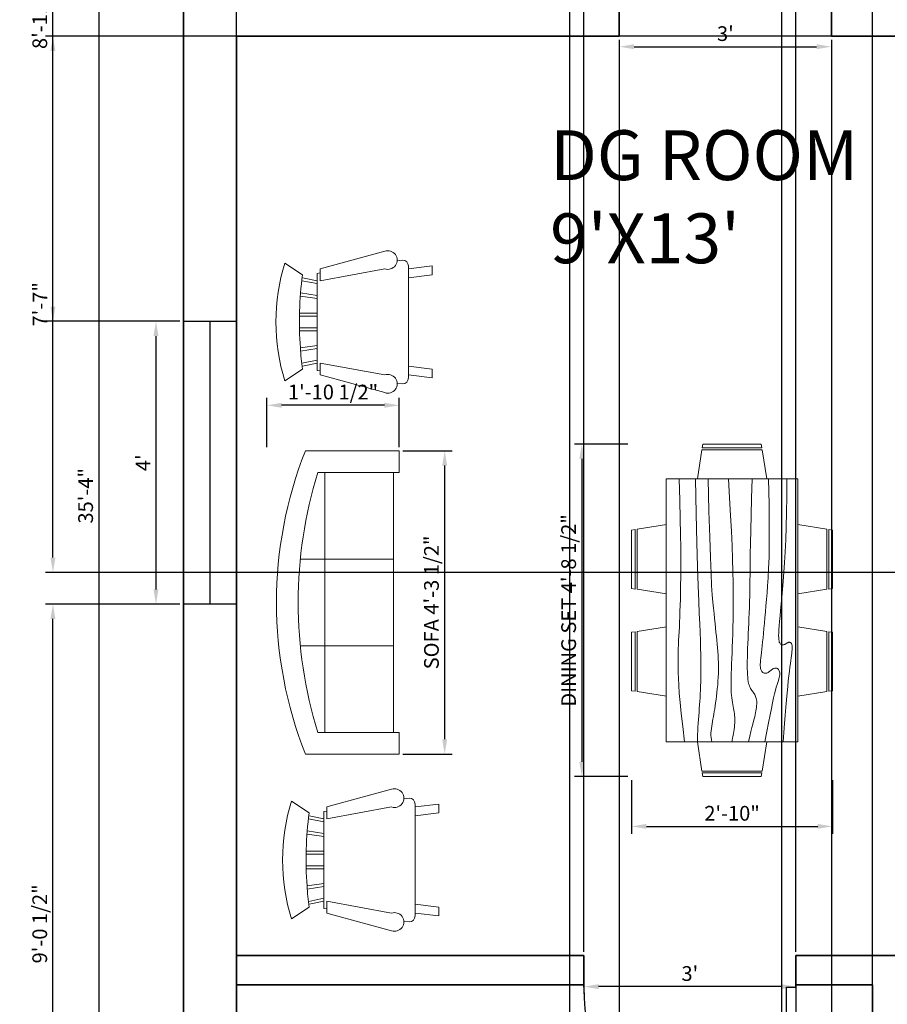
# Model space of a CAD drawing. Units: inches. Extents: x 2459 to 2755, y 1300 to 1776.
# Tile 2 of 4: x 2459 to 2606, y 1450 to 1617. Entities that reach past the tile are written whole.
import ezdxf

# ---------------------------------------------------------------- set-up
doc = ezdxf.new("R2010")
doc.units = ezdxf.units.IN
for name, color, linetype, lineweight in [('A-AREA-IDEN', 3, 'Continuous', 25), ('A-WALL', 7, 'Continuous', 35), ('DIM', 4, 'Continuous', 18), ('DOOR', 20, 'Continuous', 25), ('FURNITURE', 6, 'Continuous', 18), ('WIN', 2, 'Continuous', 25)]:
    doc.layers.add(name, color=color, linetype=linetype, lineweight=lineweight)
doc.styles.get("Standard").update_dxf_attribs({"font": 'arial.ttf'})
doc.dimstyles.new('ISO-25', dxfattribs={"dimtxt": 2.5, "dimasz": 2.5, "dimexe": 1.25, "dimexo": 0.625, "dimtad": 1, "dimlunit": 3, "dimtxsty": 'Standard', "dimcen": 2.5, "dimadec": 0, "dimazin": 0, "dimtfac": 1, "dimtmove": 0, "dimatfit": 3, "dimfxl": 1, "dimarcsym": 0})

# ---------------------------------------------------------------- blocks, each defined once
blk = doc.blocks.new('*U3')
for p, q in [((0, 0), (0, -6)), ((-40, 0), (-40, -6))]:
    blk.add_line(p, q)
blk.add_lwpolyline([(0, 0), (0, 40), (-1.75, 40), (-1.75, 0)], close=True)
blk.add_arc((0, 0), 40, 90, 180)
blk = doc.blocks.new('*U4')
for p, q in [((-40, 0), (-40, 6)), ((0, 0), (0, 6))]:
    blk.add_line(p, q)
blk.add_lwpolyline([(0, 0), (0, -40), (-1.75, -40), (-1.75, 0)], close=True)
blk.add_arc((0, 0), 40, 180, 270)
blk = doc.blocks.new('Dining Set - 36 x 72 in.')
for p, q in [((-22, 27.5), (-22.1562, 26.50042)), ((-22, 27.5), (-6, 27.5)), ((-5.8437, 26.49966), (-6, 27.5)), ((6, 27.5), (5.8438, 26.50042)), ((6, 27.5), (22, 27.5)), ((22.1563, 26.49966), (22, 27.5)), ((-22.2343, 26.00059), (-23.4847, 17.99762)), ((-22.2304, 26), (-5.7608, 26)), ((-5.8416, 26.5), (-22.1534, 26.5)), ((-4.5152, 17.99762), (-5.7655, 25.99926)), ((5.7657, 26.00059), (4.5153, 17.99762)), ((5.7696, 26), (22.2392, 26)), ((22.1584, 26.5), (5.8466, 26.5)), ((23.4848, 17.99762), (22.2345, 25.99926)), ((36, 18), (-36, 18)), ((-36, 18), (-36, -18)), ((36, -18), (36, 18)), ((-45.5, 8), (-44.5004, 8.15617)), ((-44.5, -8.15843), (-44.5, 8.15338)), ((-44.0006, 8.23428), (-35.9976, 9.48474)), ((-44, 8.23041), (-44, -8.23915)), ((44.0006, 8.23428), (35.9976, 9.48474)), ((44, 8.23041), (44, -8.23915)), ((44.5, -8.15843), (44.5, 8.15338)), ((45.5, 8), (44.5005, 8.15617)), ((-45.5, 8), (-45.5, -8)), ((45.5, 8), (45.5, -8)), ((-44.4997, -8.15631), (-45.5, -8)), ((44.4997, -8.15631), (45.5, -8)), ((-35.9976, -9.48476), (-43.9993, -8.2345)), ((35.9976, -9.48476), (43.9993, -8.2345)), ((-36, -18), (36, -18)), ((-22.2343, -26.0006), (-23.4847, -17.99762)), ((-4.5152, -17.99762), (-5.7655, -25.99928)), ((5.7657, -26.0006), (4.5153, -17.99762)), ((23.4848, -17.99762), (22.2345, -25.99928)), ((-22.2304, -26), (-5.7608, -26)), ((-22, -27.5), (-22.1562, -26.50044)), ((-5.8416, -26.5), (-22.1534, -26.5)), ((-5.8437, -26.49967), (-6, -27.5)), ((5.7696, -26), (22.2392, -26)), ((6, -27.5), (5.8438, -26.50044)), ((22.1584, -26.5), (5.8466, -26.5)), ((22.1563, -26.49967), (22, -27.5)), ((-22, -27.5), (-6, -27.5)), ((6, -27.5), (22, -27.5))]:
    blk.add_line(p, q)
for points in [[(-36, 15), (-31.1772, 14.97754), (-26.8079, 14.91406), (-22.8538, 14.81543), (-19.276, 14.6875), (-16.0362, 14.53613), (-13.0957, 14.36718), (-10.4159, 14.18652), (-7.9583, 14), (-5.6904, 13.81315), (-3.6035, 13.63021), (-1.6954, 13.45508), (0.0365, 13.29166), (1.5945, 13.14388), (2.9811, 13.01562), (4.1988, 12.9108), (5.25, 12.83333), (6.1393, 12.78613), (6.8802, 12.76823), (7.4883, 12.77767), (7.9792, 12.8125), (8.3685, 12.87077), (8.6719, 12.95052), (8.9049, 13.0498), (9.0833, 13.16666), (9.2205, 13.29899), (9.3216, 13.44401), (9.3895, 13.59879), (9.4271, 13.76041), (9.4373, 13.92594), (9.4232, 14.09245), (9.3875, 14.257), (9.3333, 14.41666), (9.2638, 14.56917), (9.1836, 14.71484), (9.0975, 14.85465), (9.0104, 14.98958), (8.9272, 15.1206), (8.8529, 15.2487), (8.7922, 15.37483), (8.75, 15.5), (8.7305, 15.62467), (8.7344, 15.74739), (8.7617, 15.86621), (8.8125, 15.97916), (8.8867, 16.08431), (8.9844, 16.17968), (9.1055, 16.26334), (9.25, 16.33333), (9.4189, 16.38802), (9.6172, 16.42708), (9.8506, 16.45052), (10.125, 16.45833), (10.4463, 16.45052), (10.8203, 16.42708), (11.2529, 16.38802), (11.75, 16.33333), (12.3184, 16.26318), (12.9694, 16.17838), (13.7151, 16.07991), (14.5677, 15.96875), (15.5395, 15.84586), (16.6426, 15.71224), (17.8893, 15.56884), (19.2917, 15.41666), (20.859, 15.25667), (22.5879, 15.08984), (24.4721, 14.91715), (26.5052, 14.73958), (28.6809, 14.5581), (30.9929, 14.3737), (33.4347, 14.18733), (36, 14)], [(-36, 10), (-28.9766, 10.14274), (-23.1725, 10.20442), (-18.4241, 10.19775), (-14.5677, 10.13541), (-11.4399, 10.03011), (-8.877, 9.89453), (-6.7154, 9.74137), (-4.7917, 9.58333), (-2.9698, 9.43082), (-1.2246, 9.28515), (0.4415, 9.14534), (2.026, 9.01041), (3.5266, 8.87939), (4.9408, 8.7513), (6.266, 8.62516), (7.5, 8.5), (8.6411, 8.37549), (9.6914, 8.2539), (10.6538, 8.13818), (11.5312, 8.03125), (12.3267, 7.93603), (13.043, 7.85547), (13.6831, 7.79248), (14.25, 7.75), (14.7471, 7.7303), (15.1797, 7.73307), (15.5537, 7.75732), (15.875, 7.80208), (16.1494, 7.86637), (16.3828, 7.94922), (16.5811, 8.04964), (16.75, 8.16666), (16.8944, 8.29915), (17.0143, 8.44531), (17.1089, 8.60319), (17.1771, 8.77083), (17.218, 8.94629), (17.2305, 9.1276), (17.2137, 9.31282), (17.1667, 9.5), (17.0895, 9.6875), (16.987, 9.875), (16.8649, 10.0625), (16.7292, 10.25), (16.5856, 10.4375), (16.4401, 10.625), (16.2985, 10.8125), (16.1667, 11), (16.05, 11.18733), (15.9518, 11.3737), (15.8752, 11.5581), (15.8229, 11.73958), (15.798, 11.91715), (15.8034, 12.08984), (15.842, 12.25667), (15.9167, 12.41666), (16.0295, 12.56836), (16.1784, 12.70833), (16.3605, 12.83268), (16.5729, 12.9375), (16.8127, 13.01888), (17.0768, 13.07291), (17.3625, 13.0957), (17.6667, 13.08333), (17.9894, 13.03312), (18.3418, 12.94726), (18.7382, 12.82918), (19.1927, 12.68229), (19.7195, 12.51001), (20.3327, 12.31575), (21.0465, 12.10294), (21.875, 11.875), (22.8357, 11.63354), (23.959, 11.37304), (25.2786, 11.08618), (26.8282, 10.76562), (28.6414, 10.40405), (30.752, 9.99414), (33.1936, 9.52856), (36, 9)], [(-36, 5.5), (-30.7157, 5.3348), (-26.069, 5.20963), (-21.9946, 5.11767), (-18.4271, 5.05208), (-15.3009, 5.00602), (-12.5508, 4.97265), (-10.1112, 4.94515), (-7.9167, 4.91666), (-5.909, 4.88167), (-4.0586, 4.83984), (-2.3429, 4.79215), (-0.7396, 4.73958), (0.7739, 4.6831), (2.22, 4.6237), (3.6213, 4.56233), (5, 4.5), (6.373, 4.43782), (7.7344, 4.3776), (9.0723, 4.32129), (10.375, 4.27083), (11.6309, 4.22819), (12.8281, 4.19531), (13.9551, 4.17415), (15, 4.16666), (15.954, 4.17448), (16.819, 4.19791), (17.6001, 4.23698), (18.3021, 4.29166), (18.9299, 4.36198), (19.4883, 4.44791), (19.9823, 4.54948), (20.4167, 4.66666), (20.7969, 4.79899), (21.1302, 4.94401), (21.4245, 5.09879), (21.6875, 5.26041), (21.9271, 5.42594), (22.1511, 5.59245), (22.3672, 5.757), (22.5834, 5.91666), (22.8065, 6.06868), (23.0404, 6.21093), (23.2879, 6.34147), (23.5521, 6.45833), (23.8358, 6.55957), (24.142, 6.64323), (24.4735, 6.70735), (24.8334, 6.75), (25.2235, 6.76969), (25.642, 6.76692), (26.0858, 6.74267), (26.5521, 6.69791), (27.0379, 6.63362), (27.5404, 6.55078), (28.0565, 6.45036), (28.5834, 6.33333), (29.1242, 6.19987), (29.7071, 6.04687), (30.3661, 5.87044), (31.1354, 5.66666), (32.0493, 5.43164), (33.142, 5.16146), (34.4475, 4.85221), (36, 4.5)], [(-36, -1), (-30.7915, -0.6591), (-26.0195, -0.38216), (-21.6519, -0.16284), (-17.6563, 0.00521), (-14.0005, 0.12833), (-10.6523, 0.21289), (-7.5796, 0.26522), (-4.75, 0.29166), (-2.134, 0.29793), (0.2878, 0.28711), (2.5317, 0.26163), (4.6146, 0.22396), (6.5529, 0.17651), (8.3633, 0.12174), (10.0623, 0.06209), (11.6667, 0), (13.1899, -0.06201), (14.6341, -0.1211), (15.9982, -0.17432), (17.2813, -0.21875), (18.4823, -0.25147), (19.6003, -0.26953), (20.6343, -0.27002), (21.5834, -0.25), (22.4481, -0.20768), (23.2357, -0.14584), (23.9549, -0.06836), (24.6146, 0.02083), (25.2235, 0.11784), (25.7904, 0.21875), (26.3241, 0.31966), (26.8334, 0.41666), (27.3265, 0.50618), (27.8099, 0.58593), (28.2894, 0.65397), (28.7709, 0.70833), (29.2601, 0.74707), (29.763, 0.76823), (30.2855, 0.76985), (30.8334, 0.75), (31.4088, 0.70784), (31.9994, 0.64713), (32.589, 0.57275), (33.1615, 0.48958), (33.7008, 0.4025), (34.1908, 0.3164), (34.6153, 0.23616), (34.9584, 0.16666), (35.2099, 0.11165), (35.3848, 0.07031), (35.504, 0.04069), (35.5886, 0.02083), (35.6594, 0.00879), (35.7377, 0.0026), (35.8442, 0.00032), (36, 0)], [(-36, -6.5), (-27.1843, -6.31267), (-20.084, -6.1263), (-14.469, -5.9419), (-10.1094, -5.76042), (-6.7752, -5.58285), (-4.2363, -5.41016), (-2.2629, -5.24333), (-0.625, -5.08334), (0.8708, -4.93099), (2.2715, -4.78646), (3.5872, -4.64974), (4.8281, -4.52084), (6.0046, -4.39974), (7.127, -4.28646), (8.2053, -4.18099), (9.25, -4.08334), (10.2705, -3.99382), (11.2734, -3.91407), (12.2647, -3.84603), (13.25, -3.79167), (14.2354, -3.75293), (15.2266, -3.73177), (16.2295, -3.73015), (17.25, -3.75), (18.2912, -3.79248), (19.3451, -3.85547), (20.4009, -3.93604), (21.4479, -4.03125), (22.4754, -4.13819), (23.4727, -4.25391), (24.4289, -4.37549), (25.3334, -4.5), (26.1785, -4.62492), (26.9694, -4.74935), (27.7145, -4.87281), (28.4219, -4.99479), (29.1, -5.11483), (29.7572, -5.23242), (30.4016, -5.34709), (31.0417, -5.45834), (31.6837, -5.56437), (32.3262, -5.65821), (32.9658, -5.73153), (33.599, -5.77604), (34.2224, -5.78345), (34.8327, -5.74545), (35.4264, -5.65373), (36, -5.5)], [(-36, -10), (-26.4022, -9.81299), (-18.4675, -9.62891), (-11.9839, -9.45069), (-6.7396, -9.28125), (-2.5226, -9.12354), (0.8789, -8.98047), (3.6769, -8.85498), (6.0833, -8.75), (8.2767, -8.66765), (10.3021, -8.60677), (12.1712, -8.56543), (13.8958, -8.54167), (15.4876, -8.53353), (16.9583, -8.53907), (18.3197, -8.55632), (19.5834, -8.58334), (20.7616, -8.61841), (21.8685, -8.66081), (22.9188, -8.71004), (23.9271, -8.76563), (24.9081, -8.82707), (25.8763, -8.89388), (26.8465, -8.96558), (27.8334, -9.04167), (28.8474, -9.12118), (29.8828, -9.20117), (30.93, -9.27824), (31.9792, -9.34896), (33.0205, -9.40991), (34.0443, -9.45768), (35.0407, -9.48885), (36, -9.5)], [(-36, -14.5), (-30.0881, -14.33513), (-25.0332, -14.21224), (-20.7312, -14.12647), (-17.0781, -14.07292), (-13.97, -14.04671), (-11.3027, -14.04297), (-8.9724, -14.05681), (-6.875, -14.08334), (-4.9224, -14.11833), (-3.0905, -14.16016), (-1.3709, -14.20785), (0.2448, -14.26042), (1.7647, -14.3169), (3.1973, -14.3763), (4.5507, -14.43767), (5.8333, -14.5), (7.0554, -14.5621), (8.235, -14.62175), (9.3922, -14.67652), (10.5469, -14.72396), (11.7192, -14.76164), (12.929, -14.78711), (14.1965, -14.79794), (15.5417, -14.79167), (16.9933, -14.76424), (18.6152, -14.70508), (20.4804, -14.60197), (22.6615, -14.44271), (25.2312, -14.21509), (28.2624, -13.9069), (31.8277, -13.50594), (36, -13)]]:
    blk.add_lwpolyline(points)
blk = doc.blocks.new('Sofa - Roundback 7 ft.')
for p, q in [((-12.00002, -32.4421), (-12.00003, -6.5971)), ((11.99997, -32.4421), (11.99998, -6.5971)), ((-36.000027, -34), (-36.000027, -11.4696)), ((-35.999844, -13.3819), (35.9998, -13.3819)), ((35.99998, -34), (35.99998, -11.4696)), ((-36.000027, -32.4421), (35.99998, -32.4421))]:
    blk.add_line(p, q)
for points in [[(-36.000027, -34), (-42.000027, -34), (-42.000027, -8)], [(41.99998, -8), (41.99998, -34), (35.99998, -34)]]:
    blk.add_lwpolyline(points)
for centre, radius, start, end in [((0, -114.25), 114.25, 68.43141, 111.5686), ((-0.00001, -127.1968), 121.1968, 72.72033, 107.2797)]:
    blk.add_arc(centre, radius, start, end)
blk = doc.blocks.new('Chair - Rocking')
for p, q in [((-8, -4.5), (-10, -1.5)), ((8, -4.5), (10, -1.5)), ((-7.5, -4.5), (-7, -7)), ((-6.5, -7), (-7.02225, -4.43)), ((-4.5, -7), (-4.96674, -4.19951)), ((-4, -7), (-4.40532, -4.16272)), ((-1.5, -4.05012), (-1.5, -7)), ((-1, -7), (-1, -4.05012)), ((1, -7), (1, -4.04655)), ((1.5, -4.05012), (1.5, -7)), ((4, -7), (4.40187, -4.18694)), ((4.5, -7), (4.96761, -4.19437)), ((6.5, -7), (7, -4.4057)), ((7.5, -4.5), (7, -7)), ((-9, -7.5), (-12, -18.49999)), ((-7, -7.5), (-9, -7.5)), ((-9, -18.49999), (-7, -7.5)), ((-8.23428, -6.99939), (-8.3093, -7.47958)), ((-8.23041, -7), (8.23915, -7)), ((7, -7.5), (9, -7.5)), ((9, -18.49999), (7, -7.5)), ((8.31071, -7.48854), (8.23449, -7.00073)), ((9, -7.5), (12, -18.49999)), ((-10.36644, -20.64523), (-10.5, -21.49999)), ((10.5, -21.49999), (10.3575, -20.58798)), ((-9, -22.49999), (-9.5, -26.49999)), ((0, -22.49999), (-9.5, -22.49999)), ((-8, -26.49999), (-7.5, -22.49999)), ((0, -22.49999), (9.5, -22.49999)), ((8, -26.49999), (7.5, -22.49999)), ((9, -22.49999), (9.5, -26.49999)), ((-9.5, -26.49999), (-8, -26.49999)), ((9.5, -26.49999), (8, -26.49999))]:
    blk.add_line(p, q)
for centre, radius, start, end in [((0, -34.08333), 34.08333, 72.93847, 107.0615), ((0, -68.25004), 64.25, 93.92211, 97.15267), ((0, -68.25004), 64.25, 82.84733, 93.92211), ((-10.5, -18.99999), 1.58114, 161.5651, 18.43495), ((10.5, -18.99999), 1.58114, 161.5651, 18.43495), ((-9.5, -21.49999), 1, 180, 270), ((9.5, -21.49999), 1, 270, 0)]:
    blk.add_arc(centre, radius, start, end)
blk = doc.blocks.new('*D19')
at = {"layer": 'Defpoints', "color": 0, "transparency": 16777216}
for p in [(2487, 1748.32), (2472.62, 1324.32), (2487, 1324.32)]:
    blk.add_point(p, dxfattribs=at)
at = {"layer": 'DIM', "color": 0, "lineweight": -2, "transparency": 16777216}
for p, q in [((2486.37, 1748.32), (2471.37, 1748.32)), ((2472.62, 1745.82), (2472.62, 1326.82)), ((2486.37, 1324.32), (2471.37, 1324.32))]:
    blk.add_line(p, q, dxfattribs=at)
at = {"layer": 'DIM', "color": 0, "transparency": 16777216}
for points in [[(2472.2, 1745.82), (2473.04, 1745.82), (2472.62, 1748.32)], [(2472.2, 1326.82), (2473.04, 1326.82), (2472.62, 1324.32)]]:
    blk.add_solid(points, dxfattribs=at)
at = {"layer": 'DIM', "color": 0, "transparency": 16777216, "insert": (2470.72, 1536.32), "char_height": 2.5, "attachment_point": 5, "rotation": 90}
blk.add_mtext('35\'-4"', dxfattribs=at)
blk = doc.blocks.new('*D21')
at = {"layer": 'Defpoints', "color": 0, "transparency": 16777216}
for p in [(2487, 1565.93), (2482.34, 1517.93), (2487, 1517.93)]:
    blk.add_point(p, dxfattribs=at)
at = {"layer": 'DIM', "color": 0, "lineweight": -2, "transparency": 16777216}
for p, q in [((2486.37, 1565.93), (2481.09, 1565.93)), ((2482.34, 1563.43), (2482.34, 1520.43)), ((2486.37, 1517.93), (2481.09, 1517.93))]:
    blk.add_line(p, q, dxfattribs=at)
at = {"layer": 'DIM', "color": 0, "transparency": 16777216}
for points in [[(2481.92, 1563.43), (2482.75, 1563.43), (2482.34, 1565.93)], [(2481.92, 1520.43), (2482.75, 1520.43), (2482.34, 1517.93)]]:
    blk.add_solid(points, dxfattribs=at)
at = {"layer": 'DIM', "color": 0, "transparency": 16777216, "insert": (2480.46, 1541.93), "char_height": 2.5, "attachment_point": 5, "rotation": 90}
blk.add_mtext("4'", dxfattribs=at)
blk = doc.blocks.new('*D22')
at = {"layer": 'Defpoints', "color": 0, "transparency": 16777216}
for p in [(2561, 1614.32), (2597, 1614.32), (2597, 1612.53)]:
    blk.add_point(p, dxfattribs=at)
at = {"layer": 'DIM', "color": 0, "lineweight": -2, "transparency": 16777216}
for p, q in [((2561, 1613.69), (2561, 1611.28)), ((2563.5, 1612.53), (2594.5, 1612.53)), ((2597, 1613.69), (2597, 1611.28))]:
    blk.add_line(p, q, dxfattribs=at)
at = {"layer": 'DIM', "color": 0, "transparency": 16777216}
for points in [[(2563.5, 1612.95), (2563.5, 1612.11), (2561, 1612.53)], [(2594.5, 1612.95), (2594.5, 1612.11), (2597, 1612.53)]]:
    blk.add_solid(points, dxfattribs=at)
at = {"layer": 'DIM', "color": 0, "transparency": 16777216, "insert": (2579, 1614.43), "char_height": 2.5, "attachment_point": 5}
blk.add_mtext("3'", dxfattribs=at)
blk = doc.blocks.new('*D31')
at = {"layer": 'Defpoints', "color": 0, "transparency": 16777216}
for p in [(2554.97, 1458.32), (2590.97, 1458.32), (2554.97, 1453.02)]:
    blk.add_point(p, dxfattribs=at)
at = {"layer": 'DIM', "color": 0, "lineweight": -2, "transparency": 16777216}
for p, q in [((2554.97, 1457.69), (2554.97, 1451.77)), ((2590.97, 1457.69), (2590.97, 1451.77)), ((2588.47, 1453.02), (2557.47, 1453.02))]:
    blk.add_line(p, q, dxfattribs=at)
at = {"layer": 'DIM', "color": 0, "transparency": 16777216}
for points in [[(2557.47, 1453.43), (2557.47, 1452.6), (2554.97, 1453.02)], [(2588.47, 1453.43), (2588.47, 1452.6), (2590.97, 1453.02)]]:
    blk.add_solid(points, dxfattribs=at)
at = {"layer": 'DIM', "color": 0, "transparency": 16777216, "insert": (2572.97, 1454.92), "char_height": 2.5, "attachment_point": 5}
blk.add_mtext("3'", dxfattribs=at)
blk = doc.blocks.new('WIN-48IN')
blk.add_line((4.5, 48), (4.5, 0))
blk.add_lwpolyline([(0, 48), (9, 48), (9, 0), (0, 0)], close=True)
blk = doc.blocks.new('*D45')
at = {"layer": 'Defpoints', "color": 0, "transparency": 16777216}
for p in [(2563.09, 1545.08), (2554.63, 1488.67), (2563.09, 1488.67)]:
    blk.add_point(p, dxfattribs=at)
at = {"layer": 'DIM', "color": 0, "lineweight": -2, "transparency": 16777216}
for p, q in [((2562.47, 1545.08), (2553.38, 1545.08)), ((2554.63, 1542.58), (2554.63, 1491.17)), ((2562.47, 1488.67), (2553.38, 1488.67))]:
    blk.add_line(p, q, dxfattribs=at)
at = {"layer": 'DIM', "color": 0, "transparency": 16777216}
for points in [[(2554.22, 1542.58), (2555.05, 1542.58), (2554.63, 1545.08)], [(2554.22, 1491.17), (2555.05, 1491.17), (2554.63, 1488.67)]]:
    blk.add_solid(points, dxfattribs=at)
at = {"layer": 'DIM', "color": 0, "transparency": 16777216, "insert": (2552.72, 1516.87), "char_height": 2.5, "attachment_point": 5, "rotation": 90}
blk.add_mtext('DINING SET 4\'-8 1/2"', dxfattribs=at)
blk = doc.blocks.new('*D46')
at = {"layer": 'Defpoints', "color": 0, "transparency": 16777216}
for p in [(2563.09, 1488.67), (2597.18, 1488.67), (2597.18, 1480.21)]:
    blk.add_point(p, dxfattribs=at)
at = {"layer": 'DIM', "color": 0, "lineweight": -2, "transparency": 16777216}
for p, q in [((2563.09, 1488.05), (2563.09, 1478.96)), ((2597.18, 1488.05), (2597.18, 1478.96)), ((2565.59, 1480.21), (2594.68, 1480.21))]:
    blk.add_line(p, q, dxfattribs=at)
at = {"layer": 'DIM', "color": 0, "transparency": 16777216}
for points in [[(2565.59, 1480.63), (2565.59, 1479.8), (2563.09, 1480.21)], [(2594.68, 1480.63), (2594.68, 1479.8), (2597.18, 1480.21)]]:
    blk.add_solid(points, dxfattribs=at)
at = {"layer": 'DIM', "color": 0, "transparency": 16777216, "insert": (2580.14, 1482.11), "char_height": 2.5, "attachment_point": 5}
blk.add_mtext('2\'-10"', dxfattribs=at)
blk = doc.blocks.new('*D47')
at = {"layer": 'Defpoints', "color": 0, "transparency": 16777216}
for p in [(2523.63, 1543.96), (2531.35, 1543.96), (2523.63, 1492.49)]:
    blk.add_point(p, dxfattribs=at)
at = {"layer": 'DIM', "color": 0, "lineweight": -2, "transparency": 16777216}
for p, q in [((2524.26, 1543.96), (2532.6, 1543.96)), ((2531.35, 1494.99), (2531.35, 1541.46)), ((2524.26, 1492.49), (2532.6, 1492.49))]:
    blk.add_line(p, q, dxfattribs=at)
at = {"layer": 'DIM', "color": 0, "transparency": 16777216}
for points in [[(2530.94, 1541.46), (2531.77, 1541.46), (2531.35, 1543.96)], [(2530.94, 1494.99), (2531.77, 1494.99), (2531.35, 1492.49)]]:
    blk.add_solid(points, dxfattribs=at)
at = {"layer": 'DIM', "color": 0, "transparency": 16777216, "insert": (2529.43, 1518.22), "char_height": 2.5, "attachment_point": 5, "rotation": 90}
blk.add_mtext('SOFA 4\'-3 1/2"', dxfattribs=at)
blk = doc.blocks.new('*D48')
at = {"layer": 'Defpoints', "color": 0, "transparency": 16777216}
for p in [(2501.17, 1551.68), (2501.17, 1543.96), (2523.63, 1543.96)]:
    blk.add_point(p, dxfattribs=at)
at = {"layer": 'DIM', "color": 0, "lineweight": -2, "transparency": 16777216}
for p, q in [((2501.17, 1544.59), (2501.17, 1552.93)), ((2523.63, 1544.59), (2523.63, 1552.93)), ((2521.13, 1551.68), (2503.67, 1551.68))]:
    blk.add_line(p, q, dxfattribs=at)
at = {"layer": 'DIM', "color": 0, "transparency": 16777216}
for points in [[(2503.67, 1552.1), (2503.67, 1551.26), (2501.17, 1551.68)], [(2521.13, 1552.1), (2521.13, 1551.26), (2523.63, 1551.68)]]:
    blk.add_solid(points, dxfattribs=at)
at = {"layer": 'DIM', "color": 0, "transparency": 16777216, "insert": (2512.4, 1553.6), "char_height": 2.5, "attachment_point": 5}
blk.add_mtext('1\'-10 1/2"', dxfattribs=at)
blk = doc.blocks.new('*D63')
at = {"layer": 'Defpoints', "color": 0, "transparency": 16777216}
for p in [(2464.85, 1517.93), (2487, 1517.93), (2487, 1409.4)]:
    blk.add_point(p, dxfattribs=at)
at = {"layer": 'DIM', "color": 0, "lineweight": -2, "transparency": 16777216}
for p, q in [((2486.37, 1517.93), (2463.6, 1517.93)), ((2464.85, 1411.9), (2464.85, 1515.43)), ((2486.37, 1409.4), (2463.6, 1409.4))]:
    blk.add_line(p, q, dxfattribs=at)
at = {"layer": 'DIM', "color": 0, "transparency": 16777216}
for points in [[(2464.43, 1515.43), (2465.26, 1515.43), (2464.85, 1517.93)], [(2464.43, 1411.9), (2465.26, 1411.9), (2464.85, 1409.4)]]:
    blk.add_solid(points, dxfattribs=at)
at = {"layer": 'DIM', "color": 0, "transparency": 16777216, "insert": (2462.93, 1463.67), "char_height": 2.5, "attachment_point": 5, "rotation": 90}
blk.add_mtext('9\'-0 1/2"', dxfattribs=at)
blk = doc.blocks.new('*D64')
at = {"layer": 'Defpoints', "color": 0, "transparency": 16777216}
for p in [(2464.85, 1673.67), (2487, 1673.67), (2487, 1565.93)]:
    blk.add_point(p, dxfattribs=at)
at = {"layer": 'DIM', "color": 0, "lineweight": -2, "transparency": 16777216}
for p, q in [((2486.37, 1673.67), (2463.6, 1673.67)), ((2464.85, 1568.43), (2464.85, 1671.17)), ((2486.37, 1565.93), (2463.6, 1565.93))]:
    blk.add_line(p, q, dxfattribs=at)
at = {"layer": 'DIM', "color": 0, "transparency": 16777216}
for points in [[(2464.43, 1671.17), (2465.26, 1671.17), (2464.85, 1673.67)], [(2464.43, 1568.43), (2465.26, 1568.43), (2464.85, 1565.93)]]:
    blk.add_solid(points, dxfattribs=at)
at = {"layer": 'DIM', "color": 0, "transparency": 16777216, "insert": (2462.93, 1619.8), "char_height": 2.5, "attachment_point": 5, "rotation": 90}
blk.add_mtext('8\'-11 1/2"', dxfattribs=at)
blk = doc.blocks.new('*D70')
at = {"layer": 'Defpoints', "color": 0, "transparency": 16777216}
for p in [(2588.61, 1770.47), (2552.61, 1374.32), (2588.61, 1374.32)]:
    blk.add_point(p, dxfattribs=at)
at = {"layer": 'DIM', "color": 0, "lineweight": -2, "transparency": 16777216}
for p, q in [((2552.61, 1374.94), (2552.61, 1771.72)), ((2588.61, 1374.94), (2588.61, 1771.72)), ((2555.11, 1770.47), (2586.11, 1770.47))]:
    blk.add_line(p, q, dxfattribs=at)
at = {"layer": 'DIM', "color": 0, "transparency": 16777216}
for points in [[(2555.11, 1770.88), (2555.11, 1770.05), (2552.61, 1770.47)], [(2586.11, 1770.88), (2586.11, 1770.05), (2588.61, 1770.47)]]:
    blk.add_solid(points, dxfattribs=at)
at = {"layer": 'DIM', "color": 0, "transparency": 16777216, "insert": (2570.61, 1772.37), "char_height": 2.5, "attachment_point": 5}
blk.add_mtext('3\'-0"', dxfattribs=at)
blk = doc.blocks.new('*D73')
at = {"layer": 'Defpoints', "color": 0, "transparency": 16777216}
for p in [(2464.85, 1614.32), (2652.14, 1614.32), (2652.14, 1523.32)]:
    blk.add_point(p, dxfattribs=at)
at = {"layer": 'DIM', "color": 0, "lineweight": -2, "transparency": 16777216}
for p, q in [((2651.52, 1614.32), (2463.6, 1614.32)), ((2464.85, 1525.82), (2464.85, 1611.82)), ((2651.52, 1523.32), (2463.6, 1523.32))]:
    blk.add_line(p, q, dxfattribs=at)
at = {"layer": 'DIM', "color": 0, "transparency": 16777216}
for points in [[(2464.43, 1611.82), (2465.26, 1611.82), (2464.85, 1614.32)], [(2464.43, 1525.82), (2465.26, 1525.82), (2464.85, 1523.32)]]:
    blk.add_solid(points, dxfattribs=at)
at = {"layer": 'DIM', "color": 0, "transparency": 16777216, "insert": (2462.97, 1568.82), "char_height": 2.5, "attachment_point": 5, "rotation": 90}
blk.add_mtext('7\'-7"', dxfattribs=at)
blk = doc.blocks.new('*D75')
at = {"layer": 'Defpoints', "color": 0, "transparency": 16777216}
for p in [(2496, 1614.32), (2561, 1614.32), (2561, 1302.17)]:
    blk.add_point(p, dxfattribs=at)
at = {"layer": 'DIM', "color": 0, "lineweight": -2, "transparency": 16777216}
for p, q in [((2496, 1613.69), (2496, 1300.92)), ((2561, 1613.69), (2561, 1300.92)), ((2498.5, 1302.17), (2558.5, 1302.17))]:
    blk.add_line(p, q, dxfattribs=at)
at = {"layer": 'DIM', "color": 0, "transparency": 16777216}
for points in [[(2498.5, 1302.58), (2498.5, 1301.75), (2496, 1302.17)], [(2558.5, 1302.58), (2558.5, 1301.75), (2561, 1302.17)]]:
    blk.add_solid(points, dxfattribs=at)
at = {"layer": 'DIM', "color": 0, "transparency": 16777216, "insert": (2528.5, 1304.06), "char_height": 2.5, "attachment_point": 5}
blk.add_mtext('5\'-5"', dxfattribs=at)
blk = doc.blocks.new('*D76')
at = {"layer": 'Defpoints', "color": 0, "transparency": 16777216}
for p in [(2597, 1614.32), (2612.48, 1614.32), (2612.48, 1302.17)]:
    blk.add_point(p, dxfattribs=at)
at = {"layer": 'DIM', "color": 0, "lineweight": -2, "transparency": 16777216}
for p, q in [((2597, 1613.69), (2597, 1300.92)), ((2612.48, 1613.69), (2612.48, 1300.92)), ((2599.5, 1302.17), (2609.98, 1302.17))]:
    blk.add_line(p, q, dxfattribs=at)
at = {"layer": 'DIM', "color": 0, "transparency": 16777216}
for points in [[(2599.5, 1302.58), (2599.5, 1301.75), (2597, 1302.17)], [(2609.98, 1302.58), (2609.98, 1301.75), (2612.48, 1302.17)]]:
    blk.add_solid(points, dxfattribs=at)
at = {"layer": 'DIM', "color": 0, "transparency": 16777216, "insert": (2604.74, 1304.09), "char_height": 2.5, "attachment_point": 5}
blk.add_mtext('1\'-3 1/2"', dxfattribs=at)
blk = doc.blocks.new('*D77')
at = {"layer": 'Defpoints', "color": 0, "transparency": 16777216}
for p in [(2554.97, 1770.47), (2496, 1458.32), (2554.97, 1458.32)]:
    blk.add_point(p, dxfattribs=at)
at = {"layer": 'DIM', "color": 0, "lineweight": -2, "transparency": 16777216}
for p, q in [((2496, 1458.94), (2496, 1771.72)), ((2554.97, 1458.94), (2554.97, 1771.72)), ((2498.5, 1770.47), (2552.47, 1770.47))]:
    blk.add_line(p, q, dxfattribs=at)
at = {"layer": 'DIM', "color": 0, "transparency": 16777216}
for points in [[(2498.5, 1770.88), (2498.5, 1770.05), (2496, 1770.47)], [(2552.47, 1770.88), (2552.47, 1770.05), (2554.97, 1770.47)]]:
    blk.add_solid(points, dxfattribs=at)
at = {"layer": 'DIM', "color": 0, "transparency": 16777216, "insert": (2525.48, 1772.35), "char_height": 2.5, "attachment_point": 5}
blk.add_mtext('4\'-11"', dxfattribs=at)
blk = doc.blocks.new('*D78')
at = {"layer": 'Defpoints', "color": 0, "transparency": 16777216}
for p in [(2610.51, 1770.47), (2590.97, 1458.32), (2610.51, 1458.32)]:
    blk.add_point(p, dxfattribs=at)
at = {"layer": 'DIM', "color": 0, "lineweight": -2, "transparency": 16777216}
for p, q in [((2590.97, 1458.94), (2590.97, 1771.72)), ((2610.51, 1458.94), (2610.51, 1771.72)), ((2593.47, 1770.47), (2608.01, 1770.47))]:
    blk.add_line(p, q, dxfattribs=at)
at = {"layer": 'DIM', "color": 0, "transparency": 16777216}
for points in [[(2593.47, 1770.88), (2593.47, 1770.05), (2590.97, 1770.47)], [(2608.01, 1770.88), (2608.01, 1770.05), (2610.51, 1770.47)]]:
    blk.add_solid(points, dxfattribs=at)
at = {"layer": 'DIM', "color": 0, "transparency": 16777216, "insert": (2600.74, 1772.38), "char_height": 2.5, "attachment_point": 5}
blk.add_mtext('1\'-7 1/2"', dxfattribs=at)
blk = doc.blocks.new('*D79')
at = {"layer": 'Defpoints', "color": 0, "transparency": 16777216}
for p in [(2604, 1770.47), (2588.61, 1374.32), (2604, 1374.32)]:
    blk.add_point(p, dxfattribs=at)
at = {"layer": 'DIM', "color": 0, "lineweight": -2, "transparency": 16777216}
for p, q in [((2588.61, 1374.94), (2588.61, 1771.72)), ((2604, 1374.94), (2604, 1771.72)), ((2591.11, 1770.47), (2601.5, 1770.47))]:
    blk.add_line(p, q, dxfattribs=at)
at = {"layer": 'DIM', "color": 0, "transparency": 16777216}
for points in [[(2591.11, 1770.88), (2591.11, 1770.05), (2588.61, 1770.47)], [(2601.5, 1770.88), (2601.5, 1770.05), (2604, 1770.47)]]:
    blk.add_solid(points, dxfattribs=at)
at = {"layer": 'DIM', "color": 0, "transparency": 16777216, "insert": (2596.3, 1772.39), "char_height": 2.5, "attachment_point": 5}
blk.add_mtext('1\'-3 1/2"', dxfattribs=at)

msp = doc.modelspace()

# ---------------------------------------------------------------- linework, layer by layer
at = {"layer": 'A-WALL'}
for p, q in [((2486.997, 1324.317), (2486.997, 1748.317)), ((2495.997, 1333.317), (2495.997, 1614.317)), ((2495.997, 1614.317), (2560.996, 1614.317)), ((2596.996, 1614.317), (2612.476, 1614.317)), ((2495.997, 1333.317), (2495.997, 1488.317)), ((2495.997, 1458.317), (2554.966, 1458.317)), ((2590.966, 1458.317), (2610.511, 1458.317)), ((2495.997, 1453.317), (2554.966, 1453.317)), ((2590.966, 1453.317), (2603.997, 1453.317)), ((2603.997, 1374.317), (2603.997, 1453.317))]:
    msp.add_line(p, q, dxfattribs=at)
for points in [[(2560.996, 1614.317), (2560.996, 1619.317)], [(2596.996, 1619.317), (2596.996, 1614.317)], [(2554.966, 1453.317), (2554.966, 1458.317)], [(2590.966, 1458.317), (2590.966, 1453.317)]]:
    msp.add_lwpolyline(points, dxfattribs=at)

# ---------------------------------------------------------------- block references
at = {"layer": 'DOOR', "xscale": 0.9, "yscale": 0.9, "zscale": 0.9}
for name, p in [('*U3', (2596.996, 1619.717)), ('*U4', (2590.966, 1452.917))]:
    msp.add_blockref(name, p, dxfattribs=at)
at = {"layer": 'FURNITURE', "rotation": 90}
for p in [(2502.699, 1565.821), (2503.831, 1474.507)]:
    msp.add_blockref('Chair - Rocking', p, dxfattribs=at)
at = {"layer": 'FURNITURE'}
for name, p, xscale, yscale, zscale, rotation in [('Dining Set - 36 x 72 in.', (2580.137, 1516.875), 0.6197986218583076, 0.6197986218583076, 0.6197986218583076, 270), ('Sofa - Roundback 7 ft.', (2502.799, 1518.225), 0.6127438370345335, 0.6127438370345335, 0.6127438370345335, 90)]:
    msp.add_blockref(name, p, dxfattribs=dict(at, xscale=xscale, yscale=yscale, zscale=zscale, rotation=rotation))
at = {"layer": 'WIN'}
msp.add_blockref('WIN-48IN', (2486.997, 1517.934), dxfattribs=at)

# ---------------------------------------------------------------- texts
at = {"layer": 'A-AREA-IDEN', "insert": (2549.242, 1598.354), "char_height": 8.4618, "attachment_point": 1}
msp.add_mtext_dynamic_manual_height_columns("{DG ROOM\\P9'X13'}", width=133.04104, gutter_width=21.155, heights=[0], dxfattribs=at)

# ---------------------------------------------------------------- dimensions: what is measured, and where the dimension line sits
at = {"layer": 'DIM'}
for base, p1, p2, override, picture, middle in [((2603.997, 1770.467), (2588.609, 1374.317), (2603.997, 1374.317), {"dimdec": 1, "dimlfac": 1, "dimrnd": 0, "dimzin": 1, "dimdsep": 46, "dimlunit": 4, "dimfrac": 2}, '*D79', (2596.303, 1772.386)), ((2610.511, 1770.467), (2590.966, 1458.317), (2610.511, 1458.317), {"dimdec": 1, "dimlfac": 1, "dimrnd": 0, "dimzin": 1, "dimdsep": 46, "dimlunit": 4, "dimfrac": 2}, '*D78', (2600.738, 1772.385)), ((2554.966, 1770.467), (2495.997, 1458.317), (2554.966, 1458.317), {"dimdec": 1, "dimlfac": 1, "dimrnd": 0, "dimzin": 1, "dimdsep": 46, "dimlunit": 4, "dimfrac": 2}, '*D77', (2525.482, 1772.347)), ((2588.609, 1770.467), (2552.609, 1374.317), (2588.609, 1374.317), {"dimdec": 1, "dimlfac": 1, "dimrnd": 0, "dimzin": 1, "dimdsep": 46, "dimlunit": 4, "dimfrac": 2}, '*D70', (2570.609, 1772.369)), ((2596.996, 1612.529), (2560.996, 1614.317), (2596.996, 1614.317), {"dimclrd": 0, "dimclre": 0, "dimclrt": 0}, '*D22', (2578.996, 1614.431)), ((2560.996, 1302.167), (2495.997, 1614.317), (2560.996, 1614.317), {"dimdec": 1, "dimlfac": 1, "dimrnd": 0, "dimzin": 1, "dimdsep": 46, "dimlunit": 4, "dimfrac": 2}, '*D75', (2528.496, 1304.063)), ((2612.476, 1302.167), (2596.996, 1614.317), (2612.476, 1614.317), {"dimdec": 1, "dimlfac": 1, "dimrnd": 0, "dimzin": 1, "dimdsep": 46, "dimlunit": 4, "dimfrac": 2}, '*D76', (2604.736, 1304.086)), ((2597.182, 1480.213), (2563.093, 1488.674), (2597.182, 1488.674), {"dimdec": 1, "dimlfac": 1, "dimrnd": 0, "dimzin": 1, "dimdsep": 46, "dimlunit": 4, "dimfrac": 2}, '*D46', (2580.137, 1482.115)), ((2554.966, 1453.016), (2590.966, 1458.317), (2554.966, 1458.317), {"dimclrd": 0, "dimclre": 0, "dimclrt": 0}, '*D31', (2572.966, 1454.918))]:
    dim = msp.add_linear_dim(base=base, p1=p1, p2=p2, dimstyle='ISO-25', override=override, dxfattribs=at)
    dim.commit()
    dim.dimension.update_dxf_attribs({"geometry": picture, "text_midpoint": middle})
for base, p1, p2, angle, override, picture, middle in [((2472.619, 1324.317), (2486.997, 1748.317), (2486.997, 1324.317), 90, {"dimclrd": 0, "dimclre": 0, "dimclrt": 0}, '*D19', (2470.717, 1536.317)), ((2464.847, 1673.674), (2486.997, 1565.934), (2486.997, 1673.674), 90, {"dimdec": 1, "dimlfac": 1, "dimrnd": 0, "dimzin": 1, "dimdsep": 46, "dimlunit": 4, "dimfrac": 2}, '*D64', (2462.929, 1619.804)), ((2464.847, 1614.317), (2652.141, 1523.317), (2652.141, 1614.317), 90, {"dimdec": 1, "dimlfac": 1, "dimrnd": 0, "dimzin": 1, "dimdsep": 46, "dimlunit": 4, "dimfrac": 2}, '*D73', (2462.972, 1568.817)), ((2482.337, 1517.934), (2486.997, 1565.934), (2486.997, 1517.934), 90, {"dimclrd": 0, "dimclre": 0, "dimclrt": 0}, '*D21', (2480.462, 1541.934)), ((2501.165, 1551.681), (2523.632, 1543.96), (2501.165, 1543.96), 180, {"dimdec": 1, "dimlfac": 1, "dimrnd": 0, "dimzin": 1, "dimdsep": 46, "dimlunit": 4, "dimfrac": 2}, '*D48', (2512.399, 1553.598)), ((2464.847, 1517.934), (2486.997, 1409.402), (2486.997, 1517.934), 90, {"dimdec": 1, "dimlfac": 1, "dimrnd": 0, "dimzin": 1, "dimdsep": 46, "dimlunit": 4, "dimfrac": 2}, '*D63', (2462.929, 1463.668))]:
    dim = msp.add_linear_dim(base=base, p1=p1, p2=p2, angle=angle, dimstyle='ISO-25', override=override, dxfattribs=at)
    dim.commit()
    dim.dimension.update_dxf_attribs({"geometry": picture, "text_midpoint": middle})
for base, p1, p2, angle, text, picture, middle in [((2554.633, 1488.674), (2563.093, 1545.075), (2563.093, 1488.674), 270, 'DINING SET <>', '*D45', (2552.715, 1516.875)), ((2531.353, 1543.96), (2523.632, 1492.49), (2523.632, 1543.96), 90, 'SOFA <>', '*D47', (2529.434, 1518.225))]:
    dim = msp.add_linear_dim(base=base, p1=p1, p2=p2, angle=angle, text=text, dimstyle='ISO-25', override={"dimdec": 1, "dimlfac": 1, "dimrnd": 0, "dimzin": 1, "dimdsep": 46, "dimlunit": 4, "dimfrac": 2}, dxfattribs=at)
    dim.commit()
    dim.dimension.update_dxf_attribs({"geometry": picture, "text_midpoint": middle})

doc.saveas('drawing.dxf')
